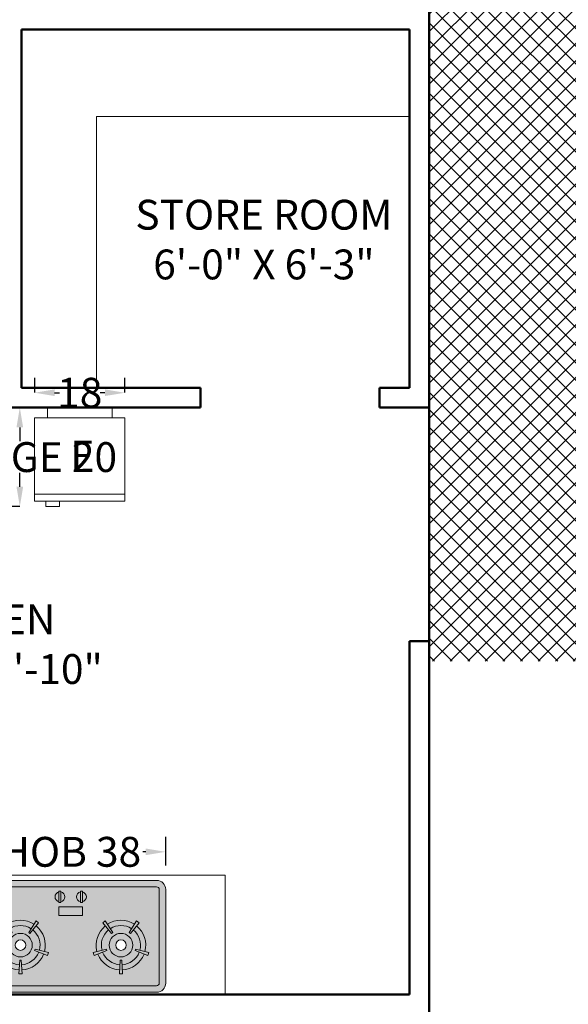
# Model space of a CAD drawing. Units: inches. Extents: x -466983 to 1020, y 324 to 318697.
# Tile 8 of 97: x 530 to 641, y 629 to 827. Entities that reach past the tile are written whole.
import ezdxf

# ---------------------------------------------------------------- set-up
doc = ezdxf.new("R2010")
doc.units = ezdxf.units.IN
doc.header["$MEASUREMENT"] = 0
for name, color, linetype, lineweight in [('A-ANNO-DIMS', 2, 'Continuous', 18), ('A-ANNO-TEXT', 7, 'Continuous', 18), ('A-AREA-IDEN', 7, 'Continuous', 25), ('A-EQPM', 8, 'Continuous', 18), ('A-FLOR-FIXT', 9, 'Continuous', 18), ('A-FLOR-PATT', 252, 'Continuous', 13), ('A-WALL', 7, 'Continuous', 50)]:
    doc.layers.add(name, color=color, linetype=linetype, lineweight=lineweight)
doc.styles.get("Standard").update_dxf_attribs({"font": 'arial.ttf'})
doc.dimstyles.get("Standard").update_dxf_attribs({"dimtxt": 6, "dimasz": 4, "dimexe": 3, "dimexo": 3, "dimgap": 0.09, "dimtad": 0, "dimtih": 1, "dimtoh": 1, "dimdec": 1, "dimzin": 0, "dimdsep": 46, "dimlunit": 3, "dimtxsty": 'Standard', "dimcen": 0.09, "dimadec": 0, "dimazin": 0, "dimtfac": 1, "dimtdec": 1, "dimtofl": 0, "dimtmove": 0, "dimatfit": 3, "dimfxl": 1, "dimtolj": 1, "dimtzin": 0, "dimarcsym": 0})

# ---------------------------------------------------------------- blocks, each defined once
blk = doc.blocks.new('Gas Stove')
h = blk.add_hatch(color=256)
h.dxf.hatch_style = 1
h.paths.add_polyline_path([(13032.81, 10915.17, 0.414214), (13029.34, 10918.64), (12963.86, 10918.64, 0.414214), (12960.39, 10915.17), (12960.39, 10879.45, 0.414214), (12963.86, 10875.98), (13029.34, 10875.98, 0.414214), (13032.81, 10879.45)])
h.paths.add_polyline_path([(13030.33, 10879.45, -0.414214), (13029.34, 10878.46), (12963.86, 10878.46, -0.414214), (12962.87, 10879.45), (12962.87, 10915.17, -0.414214), (12963.86, 10916.16), (13029.34, 10916.16, -0.414214), (13030.33, 10915.17)], flags=16)
h.paths.add_polyline_path([(13026, 10904.63), (13026.36, 10903.5), (13024.89, 10903.11, -0.295473), (13021.71, 10893.34), (13022.68, 10892.15), (13021.71, 10891.45), (13020.89, 10892.74, -0.295473), (13010.61, 10892.74), (13009.78, 10891.45), (13008.82, 10892.15), (13009.79, 10893.34, -0.295473), (13006.61, 10903.11), (13005.13, 10903.5), (13005.5, 10904.63), (13006.93, 10904.08, -0.295473), (13015.24, 10910.12), (13015.15, 10911.64), (13016.34, 10911.64), (13016.26, 10910.12, -0.295473), (13024.57, 10904.08)], flags=0)
h.paths.add_polyline_path([(13020.24, 10900.68, -1), (13011.25, 10900.68, -1)], flags=0)
h.paths.add_polyline_path([(13017.76, 10900.68, -1), (13013.73, 10900.68, -1)], flags=0)
h.paths.add_polyline_path([(13001.07, 10889.32), (13001.07, 10886.1), (12992.13, 10886.1), (12992.13, 10889.32)], flags=0)
h.paths.add_polyline_path([(13001.08, 10880.42), (13001.08, 10880.13), (13000.33, 10880.13), (13000.33, 10880.42, -0.820702), (13000.33, 10884.1), (13000.33, 10884.41), (13001.08, 10884.41), (13001.08, 10884.1, -0.816133)], flags=0)
h.paths.add_polyline_path([(12988.06, 10903.5), (12986.59, 10903.11, -0.295473), (12983.41, 10893.34), (12984.38, 10892.15), (12983.41, 10891.45), (12982.59, 10892.74, -0.295473), (12972.31, 10892.74), (12971.48, 10891.45), (12970.52, 10892.15), (12971.49, 10893.34, -0.295473), (12968.31, 10903.11), (12966.83, 10903.5), (12967.2, 10904.63), (12968.63, 10904.08, -0.295473), (12976.94, 10910.12), (12976.85, 10911.64), (12978.04, 10911.64), (12977.96, 10910.12, -0.295473), (12986.27, 10904.08), (12987.7, 10904.63)], flags=0)
h.paths.add_polyline_path([(12992.89, 10880.42), (12992.89, 10880.13), (12992.14, 10880.13), (12992.14, 10880.42, -0.816133), (12992.14, 10884.1), (12992.14, 10884.41), (12992.89, 10884.41), (12992.89, 10884.1, -0.820702)], flags=0)
h.paths.add_polyline_path([(12981.94, 10900.68, -1), (12972.95, 10900.68, -1)], flags=0)
h.paths.add_polyline_path([(12979.46, 10900.68, -1), (12975.43, 10900.68, -1)], flags=0)
h = blk.add_hatch(color=0)
h.dxf.hatch_style = 1
h.set_gradient(color1=(192, 192, 192), color2=(0, 0, 0))
h.paths.add_polyline_path([(13030.33, 10915.17, 0.414214), (13029.34, 10916.16), (12963.86, 10916.16, 0.414214), (12962.87, 10915.17), (12962.87, 10879.45, 0.414214), (12963.86, 10878.46), (13029.34, 10878.46, 0.414214), (13030.33, 10879.45)])
h.paths.add_polyline_path([(12987.7, 10904.63), (12988.06, 10903.5), (12986.59, 10903.11, -0.295473), (12983.41, 10893.34), (12984.38, 10892.15), (12983.41, 10891.45), (12982.59, 10892.74, -0.295473), (12972.31, 10892.74), (12971.48, 10891.45), (12970.52, 10892.15), (12971.49, 10893.34, -0.295473), (12968.31, 10903.11), (12966.83, 10903.5), (12967.2, 10904.63), (12968.63, 10904.08, -0.295473), (12976.94, 10910.12), (12976.85, 10911.64), (12978.04, 10911.64), (12977.96, 10910.12, -0.295473), (12986.27, 10904.08)], flags=16)
h.paths.add_polyline_path([(13005.5, 10904.63), (13006.93, 10904.08, -0.295473), (13015.24, 10910.12), (13015.15, 10911.64), (13016.34, 10911.64), (13016.26, 10910.12, -0.295473), (13024.57, 10904.08), (13026, 10904.63), (13026.36, 10903.5), (13024.89, 10903.11, -0.295473), (13021.71, 10893.34), (13022.68, 10892.15), (13021.71, 10891.45), (13020.89, 10892.74, -0.295473), (13010.61, 10892.74), (13009.78, 10891.45), (13008.82, 10892.15), (13009.79, 10893.34, -0.295473), (13006.61, 10903.11), (13005.13, 10903.5)], flags=16)
h.paths.add_polyline_path([(12981.94, 10900.68, -1), (12972.95, 10900.68, -1)], flags=0)
h.paths.add_polyline_path([(12979.46, 10900.68, -1), (12975.43, 10900.68, -1)], flags=0)
h.paths.add_polyline_path([(13020.24, 10900.68, -1), (13011.25, 10900.68, -1)], flags=0)
h.paths.add_polyline_path([(13017.76, 10900.68, -1), (13013.73, 10900.68, -1)], flags=0)
h.paths.add_polyline_path([(13001.07, 10889.32), (13001.07, 10886.1), (12992.13, 10886.1), (12992.13, 10889.32)], flags=16)
h.paths.add_polyline_path([(12992.89, 10884.41), (12992.89, 10884.1, -0.820702), (12992.89, 10880.42), (12992.89, 10880.13), (12992.14, 10880.13), (12992.14, 10880.42, -0.816133), (12992.14, 10884.1), (12992.14, 10884.41)], flags=16)
h.paths.add_polyline_path([(13000.33, 10884.41), (13001.08, 10884.41), (13001.08, 10884.1, -0.816133), (13001.08, 10880.42), (13001.08, 10880.13), (13000.33, 10880.13), (13000.33, 10880.42, -0.820702), (13000.33, 10884.1)], flags=16)
h.paths.add_polyline_path([(13022.97, 10902.61), (13021.31, 10902.17), (13021.12, 10902.73), (13022.72, 10903.36, 0.295997), (13016.14, 10908.14), (13016.04, 10906.42), (13015.45, 10906.42), (13015.35, 10908.14, 0.295997), (13008.78, 10903.36), (13010.38, 10902.73), (13010.19, 10902.17), (13008.53, 10902.61, 0.295997), (13011.04, 10894.87), (13012.13, 10896.2), (13012.61, 10895.85), (13011.68, 10894.41, 0.295997), (13019.82, 10894.41), (13018.89, 10895.85), (13019.37, 10896.2), (13020.45, 10894.87, 0.295997)], flags=0)
h = blk.add_hatch(color=256)
h.dxf.hatch_style = 1
h.set_gradient(color1=(237, 238, 153), color2=(128, 128, 128), name='INVSPHERICAL')
h.paths.add_polyline_path([(13030.33, 10915.17, 0.414214), (13029.34, 10916.16), (12963.86, 10916.16, 0.414214), (12962.87, 10915.17), (12962.87, 10879.45, 0.414214), (12963.86, 10878.46), (13029.34, 10878.46, 0.414214), (13030.33, 10879.45)])
h.paths.add_polyline_path([(12986.27, 10904.08), (12987.7, 10904.63), (12988.06, 10903.5), (12986.59, 10903.11, -0.295473), (12983.41, 10893.34), (12984.38, 10892.15), (12983.41, 10891.45), (12982.59, 10892.74, -0.295473), (12972.31, 10892.74), (12971.48, 10891.45), (12970.52, 10892.15), (12971.49, 10893.34, -0.295473), (12968.31, 10903.11), (12966.83, 10903.5), (12967.2, 10904.63), (12968.63, 10904.08, -0.295473), (12976.94, 10910.12), (12976.85, 10911.64), (12978.04, 10911.64), (12977.96, 10910.12, -0.295473)], flags=16)
h.paths.add_polyline_path([(12981.94, 10900.68, -1), (12972.95, 10900.68, -1)], flags=0)
h.paths.add_polyline_path([(12979.46, 10900.68, -1), (12975.43, 10900.68, -1)], flags=0)
h.paths.add_polyline_path([(13005.5, 10904.63), (13006.93, 10904.08, -0.295473), (13015.24, 10910.12), (13015.15, 10911.64), (13016.34, 10911.64), (13016.26, 10910.12, -0.295473), (13024.57, 10904.08), (13026, 10904.63), (13026.36, 10903.5), (13024.89, 10903.11, -0.295473), (13021.71, 10893.34), (13022.68, 10892.15), (13021.71, 10891.45), (13020.89, 10892.74, -0.295473), (13010.61, 10892.74), (13009.78, 10891.45), (13008.82, 10892.15), (13009.79, 10893.34, -0.295473), (13006.61, 10903.11), (13005.13, 10903.5)], flags=16)
h.paths.add_polyline_path([(12992.13, 10889.32), (13001.07, 10889.32), (13001.07, 10886.1), (12992.13, 10886.1)], flags=16)
h.paths.add_polyline_path([(13020.24, 10900.68, -1), (13011.25, 10900.68, -1)], flags=0)
h.paths.add_polyline_path([(13017.76, 10900.68, -1), (13013.73, 10900.68, -1)], flags=0)
h.paths.add_polyline_path([(12992.14, 10884.41), (12992.89, 10884.41), (12992.89, 10884.1, -0.820702), (12992.89, 10880.42), (12992.89, 10880.13), (12992.14, 10880.13), (12992.14, 10880.42, -0.816133), (12992.14, 10884.1)], flags=16)
h.paths.add_polyline_path([(13000.33, 10884.41), (13001.08, 10884.41), (13001.08, 10884.1, -0.816133), (13001.08, 10880.42), (13001.08, 10880.13), (13000.33, 10880.13), (13000.33, 10880.42, -0.820702), (13000.33, 10884.1)], flags=16)
h = blk.add_hatch(color=256)
h.dxf.hatch_style = 1
h.paths.add_polyline_path([(13005.5, 10904.63), (13005.13, 10903.5), (13010.19, 10902.17), (13010.38, 10902.73)])
h.paths.add_polyline_path([(13012.61, 10895.85), (13012.13, 10896.2), (13008.82, 10892.15), (13009.78, 10891.45)])
h.paths.add_polyline_path([(13019.37, 10896.2), (13018.89, 10895.85), (13021.71, 10891.45), (13022.68, 10892.15)])
h.paths.add_polyline_path([(13026.36, 10903.5), (13026, 10904.63), (13021.12, 10902.73), (13021.31, 10902.17)])
h.paths.add_polyline_path([(13016.34, 10911.64), (13015.15, 10911.64), (13015.45, 10906.42), (13016.04, 10906.42)])
h.paths.add_polyline_path([(12988.06, 10903.5), (12987.7, 10904.63), (12982.82, 10902.73), (12983.01, 10902.17)])
h.paths.add_polyline_path([(12978.04, 10911.64), (12976.85, 10911.64), (12977.15, 10906.42), (12977.74, 10906.42)])
h.paths.add_polyline_path([(12981.07, 10896.2), (12980.59, 10895.85), (12983.41, 10891.45), (12984.38, 10892.15)])
h.paths.add_polyline_path([(12974.31, 10895.85), (12973.83, 10896.2), (12970.52, 10892.15), (12971.48, 10891.45)])
h.paths.add_polyline_path([(12967.2, 10904.63), (12966.83, 10903.5), (12971.89, 10902.17), (12972.08, 10902.73)])
h = blk.add_hatch(color=256)
h.dxf.hatch_style = 1
h.paths.add_polyline_path([(12986.59, 10903.11), (12984.67, 10902.61, -0.295997), (12982.15, 10894.87), (12983.41, 10893.34, 0.295473)])
h.paths.add_polyline_path([(12977.96, 10910.12), (12977.84, 10908.14, -0.295997), (12984.42, 10903.36), (12986.27, 10904.08, 0.295473)])
h.paths.add_polyline_path([(12977.06, 10908.14), (12976.94, 10910.12, 0.295473), (12968.63, 10904.08), (12970.48, 10903.36, -0.295997)])
h.paths.add_polyline_path([(12970.23, 10902.61), (12968.31, 10903.11, 0.295473), (12971.49, 10893.34), (12972.75, 10894.87, -0.295997)])
h.paths.add_polyline_path([(12982.59, 10892.74), (12981.52, 10894.41, -0.295997), (12973.38, 10894.41), (12972.31, 10892.74, 0.295473)])
h.paths.add_polyline_path([(13016.26, 10910.12), (13016.14, 10908.14, -0.295997), (13022.72, 10903.36), (13024.57, 10904.08, 0.295473)])
h.paths.add_polyline_path([(13024.89, 10903.11), (13022.97, 10902.61, -0.295997), (13020.45, 10894.87), (13021.71, 10893.34, 0.295473)])
h.paths.add_polyline_path([(13020.89, 10892.74), (13019.82, 10894.41, -0.295997), (13011.68, 10894.41), (13010.61, 10892.74, 0.295473)])
h.paths.add_polyline_path([(13008.53, 10902.61), (13006.61, 10903.11, 0.295473), (13009.79, 10893.34), (13011.04, 10894.87, -0.295997)])
h.paths.add_polyline_path([(13015.35, 10908.14), (13015.24, 10910.12, 0.295473), (13006.93, 10904.08), (13008.78, 10903.36, -0.295997)])
h = blk.add_hatch(color=0)
h.dxf.hatch_style = 1
h.set_gradient(color1=(192, 192, 192), color2=(0, 0, 0), name='CYLINDER')
h.paths.add_polyline_path([(13022.97, 10902.61), (13021.31, 10902.17), (13021.12, 10902.73), (13022.72, 10903.36, 0.295997), (13016.14, 10908.14), (13016.04, 10906.42), (13015.45, 10906.42), (13015.35, 10908.14, 0.295997), (13008.78, 10903.36), (13010.38, 10902.73), (13010.19, 10902.17), (13008.53, 10902.61, 0.295997), (13011.04, 10894.87), (13012.13, 10896.2), (13012.61, 10895.85), (13011.68, 10894.41, 0.295997), (13019.82, 10894.41), (13018.89, 10895.85), (13019.37, 10896.2), (13020.45, 10894.87, 0.295997)])
h.paths.add_polyline_path([(13011.25, 10900.68, -1), (13020.24, 10900.68, -1)], flags=16)
h.paths.add_polyline_path([(13013.73, 10900.68, -1), (13017.76, 10900.68, -1)], flags=0)
h.paths.add_polyline_path([(12984.67, 10902.61), (12983.01, 10902.17), (12982.82, 10902.73), (12984.42, 10903.36, 0.295997), (12977.84, 10908.14), (12977.74, 10906.42), (12977.15, 10906.42), (12977.06, 10908.14, 0.295997), (12970.48, 10903.36), (12972.08, 10902.73), (12971.89, 10902.17), (12970.23, 10902.61, 0.295997), (12972.75, 10894.87), (12973.83, 10896.2), (12974.31, 10895.85), (12973.38, 10894.41, 0.295997), (12981.52, 10894.41), (12980.59, 10895.85), (12981.07, 10896.2), (12982.15, 10894.87, 0.295997)])
h.paths.add_polyline_path([(12972.95, 10900.68, -1), (12981.94, 10900.68, -1)], flags=16)
h.paths.add_polyline_path([(12975.43, 10900.68, -1), (12979.46, 10900.68, -1)], flags=0)
h = blk.add_hatch(color=0)
h.dxf.hatch_style = 1
h.set_gradient(color1=(0, 0, 255), color2=(255, 0, 0), name='CYLINDER')
h.paths.add_polyline_path([(13011.25, 10900.68, 1), (13020.24, 10900.68, 1)])
h.paths.add_polyline_path([(13017.76, 10900.68, -1), (13013.73, 10900.68, -1)], flags=16)
h.paths.add_polyline_path([(12972.95, 10900.68, 1), (12981.94, 10900.68, 1)])
h.paths.add_polyline_path([(12979.46, 10900.68, -1), (12975.43, 10900.68, -1)], flags=16)
h = blk.add_hatch(color=256)
h.dxf.hatch_style = 1
h.paths.add_polyline_path([(13001.07, 10889.32), (12992.13, 10889.32), (12992.13, 10886.1), (13001.07, 10886.1)])
h.paths.add_polyline_path([(13001.08, 10884.41), (13000.33, 10884.41), (13000.33, 10880.13), (13001.08, 10880.13)])
h.paths.add_polyline_path([(12992.89, 10884.41), (12992.14, 10884.41), (12992.14, 10880.13), (12992.89, 10880.13)])
h = blk.add_hatch(color=0)
h.dxf.hatch_style = 1
h.set_gradient(color1=(0, 0, 255), color2=(255, 0, 0), name='CYLINDER')
h.paths.add_polyline_path([(13001.08, 10884.1), (13001.08, 10880.42, 0.816133)])
h.paths.add_polyline_path([(13000.33, 10884.1, 0.820702), (13000.33, 10880.42)])
h.paths.add_polyline_path([(12992.89, 10884.1), (12992.89, 10880.42, 0.820702)])
h.paths.add_polyline_path([(12992.14, 10884.1, 0.816133), (12992.14, 10880.42)])
at = {"color": 0}
for p, q in [((12963.86, 10918.64), (13029.34, 10918.64)), ((12960.39, 10879.45), (12960.39, 10915.17)), ((12962.87, 10879.45), (12962.87, 10915.17)), ((12963.86, 10916.16), (13029.34, 10916.16)), ((13030.33, 10915.17), (13030.33, 10879.45)), ((13032.81, 10915.17), (13032.81, 10879.45)), ((12976.85, 10911.64), (12977.15, 10906.42)), ((12976.85, 10911.64), (12978.04, 10911.64)), ((12978.04, 10911.64), (12977.74, 10906.42)), ((13015.15, 10911.64), (13015.45, 10906.42)), ((13016.34, 10911.64), (13015.15, 10911.64)), ((13016.34, 10911.64), (13016.04, 10906.42)), ((12977.15, 10906.42), (12977.74, 10906.42)), ((13016.04, 10906.42), (13015.45, 10906.42)), ((12966.83, 10903.5), (12967.2, 10904.63)), ((12966.83, 10903.5), (12971.89, 10902.17)), ((12967.2, 10904.63), (12972.08, 10902.73)), ((12971.89, 10902.17), (12972.08, 10902.73)), ((12987.7, 10904.63), (12982.82, 10902.73)), ((12982.82, 10902.73), (12983.01, 10902.17)), ((12988.06, 10903.5), (12983.01, 10902.17)), ((12987.7, 10904.63), (12988.06, 10903.5)), ((13005.5, 10904.63), (13005.13, 10903.5)), ((13005.13, 10903.5), (13010.19, 10902.17)), ((13005.5, 10904.63), (13010.38, 10902.73)), ((13010.38, 10902.73), (13010.19, 10902.17)), ((13026, 10904.63), (13021.12, 10902.73)), ((13021.31, 10902.17), (13021.12, 10902.73)), ((13026.36, 10903.5), (13021.31, 10902.17)), ((13026.36, 10903.5), (13026, 10904.63)), ((12970.52, 10892.15), (12973.83, 10896.2)), ((12971.48, 10891.45), (12974.31, 10895.85)), ((12974.31, 10895.85), (12973.83, 10896.2)), ((12981.07, 10896.2), (12980.59, 10895.85)), ((12983.41, 10891.45), (12980.59, 10895.85)), ((12984.38, 10892.15), (12981.07, 10896.2)), ((13008.82, 10892.15), (13012.13, 10896.2)), ((13009.78, 10891.45), (13012.61, 10895.85)), ((13012.13, 10896.2), (13012.61, 10895.85)), ((13018.89, 10895.85), (13019.37, 10896.2)), ((13021.71, 10891.45), (13018.89, 10895.85)), ((13022.68, 10892.15), (13019.37, 10896.2)), ((12971.48, 10891.45), (12970.52, 10892.15)), ((12984.38, 10892.15), (12983.41, 10891.45)), ((13008.82, 10892.15), (13009.78, 10891.45)), ((13021.71, 10891.45), (13022.68, 10892.15)), ((12992.13, 10889.32), (12992.13, 10886.1)), ((13001.07, 10889.32), (12992.13, 10889.32)), ((13001.07, 10886.1), (13001.07, 10889.32)), ((12992.13, 10886.1), (13001.07, 10886.1)), ((12992.14, 10884.41), (12992.14, 10880.13)), ((12992.89, 10884.41), (12992.14, 10884.41)), ((12992.89, 10880.13), (12992.89, 10884.41)), ((13000.33, 10884.41), (13001.08, 10884.41)), ((13000.33, 10880.13), (13000.33, 10884.41)), ((13001.08, 10884.41), (13001.08, 10880.13)), ((12992.14, 10880.13), (12992.89, 10880.13)), ((13001.08, 10880.13), (13000.33, 10880.13)), ((13029.34, 10878.46), (12963.86, 10878.46)), ((13029.34, 10875.98), (12963.86, 10875.98))]:
    blk.add_line(p, q, dxfattribs=at)
for centre, radius in [((12977.45, 10900.68), 4.49), ((12977.45, 10900.68), 2.01), ((13015.75, 10900.68), 4.49), ((13015.75, 10900.68), 2.01)]:
    blk.add_circle(centre, radius, dxfattribs=at)
for centre, radius, start, end in [((12963.86, 10915.17), 3.47, 90, 180), ((13029.34, 10915.17), 3.47, 0, 90), ((12963.86, 10915.17), 0.992, 90, 180), ((13029.34, 10915.17), 0.992, 0, 90), ((12977.45, 10900.68), 9.46, 93.078, 158.922), ((12977.45, 10900.68), 9.46, 21.078, 86.922), ((13015.75, 10900.68), 9.46, 93.078, 158.922), ((13015.75, 10900.68), 9.46, 21.078, 86.922), ((12977.45, 10900.68), 7.47, 93.0228, 158.9772), ((12977.45, 10900.68), 7.47, 21.0228, 86.9772), ((13015.75, 10900.68), 7.47, 93.0228, 158.9772), ((13015.75, 10900.68), 7.47, 21.0228, 86.9772), ((12977.45, 10900.68), 9.46, 165.078, 230.922), ((12977.45, 10900.68), 7.47, 165.0228, 230.9772), ((12977.45, 10900.68), 7.47, 309.0228, 14.9772), ((12977.45, 10900.68), 9.46, 309.078, 14.922), ((13015.75, 10900.68), 9.46, 165.078, 230.922), ((13015.75, 10900.68), 7.47, 165.0228, 230.9772), ((13015.75, 10900.68), 7.47, 309.0228, 14.9772), ((13015.75, 10900.68), 9.46, 309.078, 14.922), ((12977.45, 10900.68), 9.46, 237.078, 302.922), ((12977.45, 10900.68), 7.47, 237.0228, 302.9772), ((13015.75, 10900.68), 9.46, 237.078, 302.922), ((13015.75, 10900.68), 7.47, 237.0228, 302.9772), ((12992.52, 10882.26), 1.88, 101.5619, 258.4381), ((12992.52, 10882.26), 1.88, 281.2484, 78.7516), ((13000.7, 10882.26), 1.88, 101.2484, 258.7516), ((13000.7, 10882.26), 1.88, 281.5619, 78.4381), ((12963.86, 10879.45), 3.47, 180, 270), ((12963.86, 10879.45), 0.992, 180, 270), ((13029.34, 10879.45), 0.992, 270, 0), ((13029.34, 10879.45), 3.47, 270, 0)]:
    blk.add_arc(centre, radius, start, end, dxfattribs=at)
blk = doc.blocks.new('A$C659B0DF6')
for p, q in [((423, 642.1), (423, 606.1)), ((513, 642.1), (423, 642.1)), ((513, 606.1), (513, 642.1)), ((585, 606.1), (0, 606.1)), ((0, 66.1), (0, 606.1)), ((585, 66.1), (585, 606.1)), ((585, 561.1), (0, 561.1)), ((0, 66.1), (585, 66.1)), ((82.3, 0), (82.3, 66.1)), ((502.7, 0), (502.7, 66.1)), ((82.3, 0), (502.7, 0))]:
    blk.add_line(p, q)
blk = doc.blocks.new('*D107')
at = {"layer": 'A-ANNO-DIMS', "color": 0, "lineweight": -2, "transparency": 16777216}
for p, q in [((521.6, 656.87), (521.6, 662.6)), ((559.81, 656.87), (559.81, 662.6)), ((525.6, 659.6), (526.23, 659.6)), ((555.81, 659.6), (555.18, 659.6))]:
    blk.add_line(p, q, dxfattribs=at)
at = {"layer": 'A-ANNO-DIMS', "color": 0, "transparency": 16777216}
for points in [[(525.6, 660.27), (525.6, 658.93), (521.6, 659.6)], [(555.81, 660.27), (555.81, 658.93), (559.81, 659.6)]]:
    blk.add_solid(points, dxfattribs=at)
at = {"layer": 'Defpoints', "color": 0, "transparency": 16777216}
for p in [(521.6, 659.6), (521.6, 653.87), (559.81, 653.87)]:
    blk.add_point(p, dxfattribs=at)
at = {"layer": 'A-ANNO-DIMS', "color": 0, "transparency": 16777216, "insert": (540.71, 659.6), "char_height": 6, "attachment_point": 5}
blk.add_mtext('\\A1;HOB 38', dxfattribs=at)
blk = doc.blocks.new('*D109')
at = {"layer": 'A-ANNO-DIMS', "color": 0, "lineweight": -2, "transparency": 16777216}
for p, q in [((530.46, 748.94), (527.47, 748.94)), ((530.47, 744.94), (530.47, 742.17)), ((530.47, 733.02), (530.47, 735.79)), ((530.46, 729.02), (527.47, 729.02))]:
    blk.add_line(p, q, dxfattribs=at)
at = {"layer": 'A-ANNO-DIMS', "color": 0, "transparency": 16777216}
for points in [[(529.8, 744.94), (531.14, 744.94), (530.47, 748.94)], [(529.8, 733.02), (531.14, 733.02), (530.47, 729.02)]]:
    blk.add_solid(points, dxfattribs=at)
at = {"layer": 'Defpoints', "color": 0, "transparency": 16777216}
for p in [(533.46, 748.94), (530.47, 729.02), (533.46, 729.02)]:
    blk.add_point(p, dxfattribs=at)
at = {"layer": 'A-ANNO-DIMS', "color": 0, "transparency": 16777216, "insert": (530.47, 738.98), "char_height": 6, "attachment_point": 5}
blk.add_mtext('\\A1;FRIDGE 20', dxfattribs=at)
blk = doc.blocks.new('*D110')
at = {"layer": 'A-ANNO-DIMS', "color": 0, "lineweight": -2, "transparency": 16777216}
for p, q in [((533.46, 751.94), (533.46, 754.92)), ((551.6, 751.94), (551.6, 754.92)), ((537.46, 751.92), (538.42, 751.92)), ((547.6, 751.92), (546.64, 751.92))]:
    blk.add_line(p, q, dxfattribs=at)
at = {"layer": 'A-ANNO-DIMS', "color": 0, "transparency": 16777216}
for points in [[(537.46, 752.59), (537.46, 751.26), (533.46, 751.92)], [(547.6, 752.59), (547.6, 751.26), (551.6, 751.92)]]:
    blk.add_solid(points, dxfattribs=at)
at = {"layer": 'Defpoints', "color": 0, "transparency": 16777216}
for p in [(533.46, 751.92), (533.46, 748.94), (551.6, 748.94)]:
    blk.add_point(p, dxfattribs=at)
at = {"layer": 'A-ANNO-DIMS', "color": 0, "transparency": 16777216, "insert": (542.53, 751.92), "char_height": 6, "attachment_point": 5}
blk.add_mtext('\\A1;18', dxfattribs=at)

msp = doc.modelspace()

# ---------------------------------------------------------------- hatches: boundary and pattern name
at = {"layer": 'A-FLOR-PATT', "transparency": 33554572}
h = msp.add_hatch(dxfattribs=at)
h.set_pattern_fill('ANSI37', color=256, scale=30)
h.set_pattern_definition([(45, (-1212.4137, -290.035), (-2.6516504, 2.6516504), []), (135, (-1212.4137, -290.035), (-2.6516504, -2.6516504), [])])
h.paths.add_polyline_path([(901.81, 1075.94), (900.61, 1075.94), (900.61, 1065.39), (899.39, 1065.39), (898.09, 1065.39), (892.84, 1058.71, -0.258377), (892.19, 1058.35), (879.98, 1058.35, -0.20177), (879.44, 1058.58), (874.08, 1065.39), (872.78, 1065.39), (871.56, 1065.39), (871.56, 1075.94), (813.81, 1075.94), (813.81, 1044.79), (832.39, 1044.79, -0.394795), (848.66, 1028.54), (848.66, 1009.94), (901.81, 1009.94), (901.81, 1015.94), (901.31, 1015.94), (871.31, 1015.94), (871.31, 1017.25), (871.33, 1017.25, -0.401453), (901.31, 1045.94), (901.81, 1045.94)])
edge = h.paths.add_edge_path(flags=16)
edge.add_line((847.77, 1068.95), (847.77, 1073.71))
edge.add_arc((849.23, 1073.71), 1.45, 90, 180, ccw=False)
edge.add_line((849.23, 1075.16), (864.49, 1075.16))
edge.add_arc((864.49, 1073.71), 1.45, 0, 90, ccw=False)
edge.add_line((865.95, 1073.71), (865.95, 1069))
edge.add_arc((832.64, 1068.98), 33.3, -20.6123, 0.0472, ccw=False)
edge.add_ellipse((856.86, 1058.48), major_axis=(0, 10.21), ratio=0.685919, start_angle=100.0088, end_angle=259.9912, ccw=False)
edge.add_arc((881.07, 1068.98), 33.3, 180.0472, 200.6123, ccw=False)
h.paths.add_polyline_path([(853.15, 1066.48), (853.15, 1066.45), (853.15, 1066.45, 0.433107), (852.92, 1066.68), (852.92, 1066.45), (853.15, 1066.45), (853.15, 1066.48), (853.09, 1066.61, 0.697939), (852.7, 1066.45), (852.7, 1066.45), (852.7, 1066.48), (852.92, 1067), (852.92, 1066.68, -0.396254)], flags=0)
h.paths.add_polyline_path([(861.02, 1066.48), (861.02, 1066.45), (861.02, 1066.45, 0.416404), (860.8, 1066.68), (860.8, 1066.45), (861.02, 1066.45), (861.02, 1066.48), (860.97, 1066.61, 0.713344), (860.57, 1066.45), (860.57, 1066.45), (860.57, 1066.48), (860.8, 1067), (860.8, 1066.68, -0.379973)], flags=0)
edge = h.paths.add_edge_path(flags=0)
edge.add_spline(control_points=[(861.13, 1065.79), (861.47, 1065.25), (861.61, 1065.02), (861.98, 1064.37), (862.19, 1063.94), (862.56, 1063.04), (862.72, 1062.56), (862.99, 1061.58), (863.09, 1061.07), (863.25, 1060.03), (863.29, 1059.5), (863.33, 1058.44), (863.32, 1057.91), (863.24, 1056.85), (863.17, 1056.33), (862.97, 1055.31), (862.84, 1054.81), (862.54, 1053.85), (862.36, 1053.39), (861.95, 1052.52), (861.73, 1052.12), (861.23, 1051.36), (860.97, 1051.02), (860.4, 1050.39), (860.11, 1050.12), (859.49, 1049.65), (859.18, 1049.45), (858.53, 1049.13), (858.2, 1049.01), (857.53, 1048.85), (857.2, 1048.81), (856.52, 1048.81), (856.19, 1048.85), (855.52, 1049.01), (855.19, 1049.13), (854.54, 1049.45), (854.23, 1049.64), (853.61, 1050.12), (853.32, 1050.39), (852.75, 1051.01), (852.49, 1051.36), (852, 1052.11), (851.77, 1052.52), (851.36, 1053.39), (851.18, 1053.85), (850.88, 1054.81), (850.75, 1055.31), (850.55, 1056.33), (850.48, 1056.85), (850.4, 1057.9), (850.39, 1058.44), (850.43, 1059.5), (850.47, 1060.03), (850.63, 1061.07), (850.73, 1061.58), (851, 1062.56), (851.16, 1063.04), (851.53, 1063.94), (851.73, 1064.37), (852.11, 1065.02), (852.25, 1065.25), (852.61, 1065.73)], knot_values=[3.915332, 3.915332, 3.915332, 3.915332, 4.013468, 4.013468, 4.175532, 4.175532, 4.337596, 4.337596, 4.49966, 4.49966, 4.661724, 4.661724, 4.823788, 4.823788, 4.985852, 4.985852, 5.147916, 5.147916, 5.30998, 5.30998, 5.472044, 5.472044, 5.634109, 5.634109, 5.796173, 5.796173, 5.958237, 5.958237, 6.120301, 6.120301, 6.282365, 6.282365, 6.444429, 6.444429, 6.606493, 6.606493, 6.768557, 6.768557, 6.930621, 6.930621, 7.092685, 7.092685, 7.254749, 7.254749, 7.416813, 7.416813, 7.578878, 7.578878, 7.740942, 7.740942, 7.903006, 7.903006, 8.06507, 8.06507, 8.227134, 8.227134, 8.389198, 8.389198, 8.551262, 8.551262, 8.65037, 8.65037, 8.65037, 8.65037], degree=3, periodic=0)
edge.add_line((852.64, 1065.79), (861.13, 1065.79))
edge = h.paths.add_edge_path(flags=0)
edge.add_ellipse((856.85, 1057.74), major_axis=(0, 7.79), ratio=0.687861, start_angle=0, end_angle=360)
h.paths.add_polyline_path([(848.86, 1069.39), (848.86, 1073.96, -0.414214), (849.95, 1075.05), (863.77, 1075.05, -0.414214), (864.86, 1073.96), (864.86, 1069.39, -0.388936), (864.52, 1069.03, -0.043561), (849.2, 1069.03, -0.388936)], flags=0)
h.paths.add_polyline_path([(853.1, 1068.11, -1), (852.68, 1068.11, -1)], flags=0)
edge = h.paths.add_edge_path(flags=0)
edge.add_ellipse((856.86, 1057.34), major_axis=(0, 2.21), ratio=0.657164, start_angle=0, end_angle=360)
h.paths.add_polyline_path([(861.04, 1068.11, -1), (860.62, 1068.11, -1)], flags=0)
edge = h.paths.add_edge_path()
edge.add_line((573.95, 1057.34), (573.95, 1075.94))
edge.add_line((573.95, 1075.94), (558.73, 1075.94))
edge.add_line((558.73, 1075.94), (558.73, 1065.39))
edge.add_line((558.73, 1065.39), (557.51, 1065.39))
edge.add_line((557.51, 1065.39), (556.21, 1065.39))
edge.add_line((556.21, 1065.39), (550.95, 1058.71))
edge.add_arc((550.3, 1059.12), 0.765, 270, 327.9483, ccw=False)
edge.add_line((550.3, 1058.35), (538.1, 1058.35))
edge.add_arc((538.1, 1059.12), 0.765, 224.3704, 270, ccw=False)
edge.add_line((537.55, 1058.58), (532.2, 1065.39))
edge.add_line((532.2, 1065.39), (530.9, 1065.39))
edge.add_line((530.9, 1065.39), (529.67, 1065.39))
edge.add_line((529.67, 1065.39), (529.67, 1075.94))
edge.add_line((529.67, 1075.94), (520.81, 1075.94))
edge.add_line((520.81, 1075.94), (520.81, 1045.94))
edge.add_line((520.81, 1045.94), (521.31, 1045.94))
edge.add_arc((521.31, 1015.94), 30, 2.5075, 90, ccw=False)
edge.add_line((551.28, 1017.25), (551.31, 1017.25))
edge.add_line((551.31, 1017.25), (551.31, 1015.94))
edge.add_line((551.31, 1015.94), (520.81, 1015.94))
edge.add_line((520.81, 1015.94), (520.81, 1009.94))
edge.add_line((520.81, 1009.94), (559.19, 1010.4))
edge.add_arc((559.19, 1011.86), 1.45, 180, 270, ccw=False)
edge.add_line((557.74, 1011.86), (557.74, 1016.56))
edge.add_arc((591.04, 1016.59), 33.3, 159.3877, 180.0472, ccw=False)
edge.add_ellipse((566.82, 1027.08), major_axis=(0, 10.21), ratio=0.685919, start_angle=280.0088, end_angle=439.9912, ccw=False)
edge.add_arc((542.61, 1016.59), 33.3, 0.0472, 20.6123, ccw=False)
edge.add_line((575.91, 1016.62), (575.91, 1011.86))
edge.add_arc((574.46, 1011.86), 1.45, -90, 0, ccw=False)
edge.add_line((574.46, 1010.4), (608.81, 1009.94))
edge.add_line((608.81, 1009.94), (608.81, 1041.09))
edge.add_line((608.81, 1041.09), (590.22, 1041.09))
edge.add_arc((590.78, 1057.91), 16.83, 181.9277, 268.1032, ccw=False)
edge = h.paths.add_edge_path()
edge.add_ellipse((494.24, 583.62), major_axis=(0, 10.21), ratio=0.685919, start_angle=280.0088, end_angle=439.9912, ccw=False)
edge.add_arc((470.03, 573.12), 33.3, 0.0472, 20.6123, ccw=False)
edge.add_line((503.33, 573.15), (503.33, 568.39))
edge.add_arc((501.88, 568.39), 1.45, -90, 0, ccw=False)
edge.add_line((501.88, 566.94), (539.81, 566.94))
edge.add_line((539.81, 566.94), (539.81, 572.94))
edge.add_line((539.81, 572.94), (539.31, 572.94))
edge.add_line((539.31, 572.94), (509.31, 572.94))
edge.add_line((509.31, 572.94), (509.31, 574.25))
edge.add_line((509.31, 574.25), (509.33, 574.25))
edge.add_arc((539.31, 572.94), 30, 90, 177.4925, ccw=False)
edge.add_line((539.31, 602.94), (539.81, 602.94))
edge.add_line((539.81, 602.94), (539.81, 626.94))
edge.add_line((539.81, 626.94), (531.77, 626.94))
edge.add_line((531.77, 626.94), (531.77, 616.39))
edge.add_line((531.77, 616.39), (530.55, 616.39))
edge.add_line((530.55, 616.39), (529.25, 616.39))
edge.add_line((529.25, 616.39), (523.71, 609.35))
edge.add_line((523.71, 609.35), (510.78, 609.35))
edge.add_line((510.78, 609.35), (505.24, 616.39))
edge.add_line((505.24, 616.39), (503.94, 616.39))
edge.add_line((503.94, 616.39), (502.72, 616.39))
edge.add_line((502.72, 616.39), (502.72, 626.94))
edge.add_line((502.72, 626.94), (481.7, 626.94))
edge.add_line((481.7, 626.94), (481.7, 611))
edge.add_arc((467.27, 611.47), 14.44, 271.9277, 358.1032, ccw=False)
edge.add_line((467.76, 597.05), (451.81, 597.05))
edge.add_line((451.81, 597.05), (451.81, 584.4))
edge.add_line((451.81, 584.4), (451.81, 566.94))
edge.add_line((451.81, 566.94), (486.61, 566.94))
edge.add_arc((486.61, 568.39), 1.45, 180, 270, ccw=False)
edge.add_line((485.16, 568.39), (485.16, 573.1))
edge.add_arc((518.46, 573.12), 33.3, 159.3877, 180.0472, ccw=False)
h.paths.add_polyline_path([(836.26, 1020.73), (879.89, 1020.73), (879.89, 1039.39), (836.26, 1039.39)], flags=25)
h.paths.add_polyline_path([(549.99, 1036.75), (593.61, 1036.75), (593.61, 1055.41), (549.99, 1055.41)], flags=24)
h.paths.add_polyline_path([(475.12, 595.6), (518.75, 595.6), (518.75, 614.25), (475.12, 614.25)], flags=24)
h = msp.add_hatch(dxfattribs=at)
h.set_pattern_fill('ANSI37', color=256, scale=20)
h.set_pattern_definition([(45, (-1212.4137, -290.035), (-1.767767, 1.767767), []), (135, (-1212.4137, -290.035), (-1.767767, -1.767767), [])])
h.paths.add_polyline_path([(809.81, 870.94), (809.81, 888.15), (807, 888.15), (802.66, 888.15), (789.38, 888.15), (786.28, 888.15, -0.414214), (785.5, 888.94), (785.5, 900.2), (785.5, 908.47, -0.414214), (786.81, 909.78, -0.414214), (785.5, 911.09), (785.5, 929.1, -0.414214), (786.81, 930.41, -0.414214), (785.5, 931.72), (785.5, 931.9, -0.414214), (784.19, 930.59), (766.72, 930.59, -0.412359), (765.41, 931.9, -0.413741), (764.11, 930.58), (744.58, 930.42, -0.416556), (743.79, 931.21), (743.79, 933.52), (742.22, 933.52), (742.22, 952.02, -0.001344), (743.79, 952.2), (743.79, 953.94), (678.59, 953.94), (678.59, 951.13), (678.59, 946.79), (678.59, 933.52), (678.59, 930.42, -0.414214), (677.81, 929.63), (666.55, 929.63), (658.27, 929.63, -0.414214), (656.96, 930.94, -0.414214), (655.66, 929.63), (637.64, 929.63, -0.414214), (636.33, 930.94, -0.414214), (635.02, 929.63), (634.84, 929.63, -0.414214), (636.15, 928.32), (636.15, 910.85, -0.412359), (634.85, 909.55, -0.413741), (636.17, 908.25), (636.32, 888.71, -0.416556), (635.54, 887.92), (633.23, 887.92), (633.23, 886.35), (614.72, 886.35, -0.001344), (614.54, 887.92), (612.81, 887.92), (612.81, 834.94), (612.81, 752.94), (612.81, 748.94), (612.81, 697.94), (654.81, 697.94), (654.81, 701.94), (715.81, 701.94), (715.81, 737.44), (774.29, 737.44), (774.29, 795.94), (809.81, 795.94)])
h.paths.add_polyline_path([(679.28, 849.58, 0.102523), (682.15, 849.26, -0.080461), (694.54, 849.77, -0.283899), (694.48, 849.01, 0.136605), (694.41, 848.81, -0.030441), (694.54, 846.89), (694.54, 842.62), (694.54, 838.35, -0.028219), (694.42, 836.57), (694.43, 836.57, 0.196187), (694.45, 836.27, -0.302897), (694.54, 835.47, -0.080461), (682.15, 835.98, 0.102523), (679.28, 835.66, -0.58611), (678.65, 836.02), (678.65, 849.22, -0.58611)], flags=16)
h.paths.add_polyline_path([(679.52, 848.65, 0.699597), (679.48, 848.63, 1.20716), (679.19, 848.74, 0.010621)], flags=0)
h.paths.add_polyline_path([(679.49, 836.56, -0.013798), (679.92, 836.66, -0.071703), (682.85, 837.14, -0.165743), (682.17, 839.1), (682.17, 842.61), (682.17, 846.06, -0.240616), (683.47, 848.68, -0.068263), (693.93, 849.01), (693.79, 848.71), (693.79, 849.02, 0.067332), (683.47, 848.68, 0.240616), (682.17, 846.06), (682.17, 842.61), (682.17, 839.1, 0.23459), (683.46, 836.55, 0.068093), (693.79, 836.2), (693.79, 836.51), (693.93, 836.21, -0.077215), (682.24, 836.78, 0.086627), (679.53, 836.57, -0.628402), (679.5, 836.57), (679.5, 836.61, 0.910458)], flags=0)
h.paths.add_polyline_path([(679.48, 848.64), (679.21, 848.65), (679.21, 836.57, 0.913566), (679.36, 836.59), (679.48, 836.58)], flags=0)
h.paths.add_polyline_path([(679.28, 829.86, 0.102523), (682.15, 829.55, -0.080461), (694.54, 830.06, -0.283899), (694.48, 829.29, 0.136605), (694.41, 829.1, -0.030441), (694.54, 827.18), (694.54, 822.9), (694.54, 818.63, -0.028219), (694.42, 816.85), (694.43, 816.85, 0.196187), (694.45, 816.56, -0.302897), (694.54, 815.75, -0.080461), (682.15, 816.26, 0.102523), (679.28, 815.95, -0.58611), (678.65, 816.3), (678.65, 829.51, -0.58611)], flags=16)
h.paths.add_polyline_path([(679.52, 828.94, 0.699597), (679.48, 828.92, 1.20716), (679.19, 829.03, 0.010621)], flags=0)
h.paths.add_polyline_path([(679.49, 816.85, -0.013798), (679.92, 816.94, -0.071703), (682.85, 817.43, -0.165743), (682.17, 819.39), (682.17, 822.89), (682.17, 826.34, -0.240616), (683.47, 828.96, -0.068263), (693.93, 829.29), (693.79, 828.99), (693.79, 829.31, 0.067332), (683.47, 828.96, 0.240616), (682.17, 826.34), (682.17, 822.89), (682.17, 819.39, 0.23459), (683.46, 816.84, 0.068093), (693.79, 816.48), (693.79, 816.8), (693.93, 816.49, -0.077215), (682.24, 817.07, 0.086627), (679.53, 816.85, -0.628402), (679.5, 816.86), (679.5, 816.89, 0.910458)], flags=0)
h.paths.add_polyline_path([(679.48, 828.92), (679.21, 828.93), (679.21, 816.86, 0.913566), (679.36, 816.87), (679.48, 816.87)], flags=0)
h.paths.add_polyline_path([(679.28, 810.15, 0.102523), (682.15, 809.83, -0.080461), (694.54, 810.34, -0.3023), (694.45, 809.54, 0.10023), (694.41, 809.39, -0.03057), (694.54, 807.46), (694.54, 803.19), (694.54, 798.92, -0.03057), (694.41, 796.99, 0.10023), (694.45, 796.84, -0.3023), (694.54, 796.04, -0.080461), (682.15, 796.55, 0.102523), (679.28, 796.23, -0.58611), (678.65, 796.59), (678.65, 809.79, -0.58611)], flags=16)
h.paths.add_polyline_path([(679.52, 809.24, 0.699597), (679.48, 809.22, 1.20716), (679.19, 809.33, 0.010621)], flags=0)
h.paths.add_polyline_path([(679.49, 797.15, -0.013798), (679.92, 797.25, -0.071703), (682.85, 797.73, -0.165743), (682.17, 799.69), (682.17, 803.2), (682.17, 806.65, -0.239349), (683.46, 809.26, -0.072465), (694.45, 809.54, 0.197932), (694.43, 809.24), (693.79, 809.3), (693.79, 809.61, 0.068093), (683.46, 809.26, 0.239349), (682.17, 806.65), (682.17, 803.2), (682.17, 799.69, 0.235854), (683.47, 797.13, 0.067332), (693.79, 796.79), (693.79, 797.1), (694.43, 797.16, 0.197932), (694.45, 796.86, -0.080419), (682.16, 797.38, 0.083867), (679.53, 797.16, -0.628402), (679.5, 797.16), (679.5, 797.2, 0.910458)], flags=0)
h.paths.add_polyline_path([(679.21, 809.24), (679.21, 797.16, 0.913566), (679.36, 797.18), (679.48, 797.17), (679.48, 809.23)], flags=0)
h.paths.add_polyline_path([(695.36, 853.3), (728.22, 853.3), (728.22, 771.15), (695.36, 771.15)], flags=16)
h.paths.add_polyline_path([(696.02, 852.64), (727.57, 852.64), (727.57, 771.81), (696.02, 771.81)], flags=0)
h.paths.add_polyline_path([(679.28, 788.79, 0.102523), (682.15, 788.47, -0.080461), (694.54, 788.98, -0.3023), (694.45, 788.18, 0.10023), (694.41, 788.03, -0.03057), (694.54, 786.1), (694.54, 781.83), (694.54, 777.56, -0.03057), (694.41, 775.63, 0.10023), (694.45, 775.48, -0.3023), (694.54, 774.68, -0.080461), (682.15, 775.19, 0.102523), (679.28, 774.88, -0.58611), (678.65, 775.23), (678.65, 788.43, -0.58611)], flags=16)
h.paths.add_polyline_path([(679.52, 787.88, 0.699597), (679.48, 787.87, 1.20716), (679.19, 787.97, 0.010621)], flags=0)
h.paths.add_polyline_path([(679.49, 775.79, -0.013798), (679.92, 775.89, -0.071703), (682.85, 776.38, -0.165743), (682.17, 778.33), (682.17, 781.84), (682.17, 785.29, -0.239349), (683.46, 787.9, -0.072465), (694.45, 788.18, 0.197932), (694.43, 787.88), (693.79, 787.94), (693.79, 788.26, 0.068093), (683.46, 787.9, 0.239349), (682.17, 785.29), (682.17, 781.84), (682.17, 778.33, 0.235854), (683.47, 775.77, 0.067332), (693.79, 775.43), (693.79, 775.74), (694.43, 775.8, 0.197932), (694.45, 775.5, -0.080419), (682.16, 776.02, 0.083867), (679.53, 775.8, -0.628402), (679.5, 775.81), (679.5, 775.84, 0.910458)], flags=0)
h.paths.add_polyline_path([(679.21, 787.88), (679.21, 775.8, 0.913566), (679.36, 775.82), (679.48, 775.81), (679.48, 787.87)], flags=0)
h.paths.add_polyline_path([(704.64, 854.12, -0.080461), (705.15, 866.52, 0.102523), (704.84, 869.39, -0.58611), (705.19, 870.02), (718.4, 870.02, -0.58611), (718.75, 869.39, 0.102523), (718.43, 866.52, -0.080461), (718.95, 854.12, -0.3023), (718.14, 854.22, 0.10023), (717.99, 854.26, -0.03057), (716.07, 854.12), (711.79, 854.12), (707.52, 854.12, -0.03057), (705.6, 854.26, 0.10023), (705.44, 854.22, -0.3023)], flags=16)
h.paths.add_polyline_path([(717.85, 869.15, 0.699597), (717.83, 869.19, 1.20716), (717.94, 869.47, 0.010621)], flags=0)
h.paths.add_polyline_path([(705.46, 854.22, -0.080419), (705.98, 866.51, 0.083867), (705.76, 869.13, -0.628402), (705.77, 869.16), (705.8, 869.16, 0.910458), (705.76, 869.17, -0.013798), (705.85, 868.75, -0.071703), (706.34, 865.81, -0.165743), (708.3, 866.5), (711.8, 866.5), (715.25, 866.5, -0.239349), (717.86, 865.2, -0.072465), (718.15, 854.22, 0.197932), (717.85, 854.24), (717.9, 854.88), (718.22, 854.88, 0.068093), (717.86, 865.2, 0.239349), (715.25, 866.5), (711.8, 866.5), (708.3, 866.5, 0.235854), (705.74, 865.19, 0.067332), (705.39, 854.88), (705.71, 854.88), (705.76, 854.24, 0.197932)], flags=16)
h.paths.add_polyline_path([(705.77, 869.46, 0.913566), (705.78, 869.3), (705.78, 869.19), (717.83, 869.19), (717.84, 869.46)], flags=0)
h.paths.add_polyline_path([(729.04, 842.62), (729.04, 846.89, -0.03057), (729.18, 848.82, 0.10023), (729.14, 848.97, -0.3023), (729.04, 849.77, -0.080461), (741.44, 849.26, 0.102523), (744.31, 849.58, -0.58611), (744.94, 849.22), (744.94, 836.02, -0.58611), (744.31, 835.66, 0.102523), (741.44, 835.98, -0.080461), (729.04, 835.47, -0.3023), (729.14, 836.27, 0.10023), (729.18, 836.42, -0.03057), (729.04, 838.35)], flags=16)
h.paths.add_polyline_path([(744.11, 836.58, 1.20716), (744.39, 836.48, 0.010621), (744.07, 836.57, 0.699597)], flags=0)
h.paths.add_polyline_path([(729.14, 836.27, 0.197932), (729.16, 836.57), (729.8, 836.51), (729.8, 836.2, 0.068093), (740.13, 836.55, 0.239349), (741.42, 839.16), (741.42, 842.61), (741.42, 846.12, 0.235854), (740.11, 848.68, 0.067332), (729.8, 849.02), (729.8, 848.71), (729.16, 848.65, 0.197932), (729.14, 848.95, -0.080419), (741.43, 848.43, 0.083867), (744.06, 848.65, -0.628402), (744.08, 848.65), (744.08, 848.61, 0.910458), (744.1, 848.66, -0.013798), (743.67, 848.56, -0.071703), (740.73, 848.08, -0.165743), (741.42, 846.12), (741.42, 842.61), (741.42, 839.16, -0.239349), (740.13, 836.55, -0.072465)], flags=0)
h.paths.add_polyline_path([(729.04, 830.06, -0.080461), (741.44, 829.55, 0.102523), (744.31, 829.86, -0.58611), (744.94, 829.51), (744.94, 816.3, -0.58611), (744.31, 815.95, 0.102523), (741.44, 816.26, -0.080461), (729.04, 815.75, -0.3023), (729.14, 816.55, 0.10023), (729.18, 816.71, -0.03057), (729.04, 818.63), (729.04, 822.9), (729.04, 827.18, -0.03057), (729.18, 829.1, 0.10023), (729.14, 829.25, -0.3023)], flags=16)
h.paths.add_polyline_path([(744.11, 816.87, 1.20716), (744.39, 816.76, 0.010621), (744.07, 816.85, 0.699597)], flags=0)
h.paths.add_polyline_path([(729.14, 829.24, -0.080419), (741.43, 828.71, 0.083867), (744.06, 828.93, -0.628402), (744.08, 828.93), (744.08, 828.9, 0.910458), (744.1, 828.94, -0.013798), (743.67, 828.84, -0.071703), (740.73, 828.36, -0.165743), (741.42, 826.4), (741.42, 822.89), (741.42, 819.44, -0.239349), (740.13, 816.84, -0.072465), (729.14, 816.55, 0.197932), (729.16, 816.85), (729.8, 816.8), (729.8, 816.48, 0.068093), (740.13, 816.84, 0.239349), (741.42, 819.44), (741.42, 822.89), (741.42, 826.4, 0.235854), (740.11, 828.96, 0.067332), (729.8, 829.31), (729.8, 828.99), (729.16, 828.94, 0.197932)], flags=16)
h.paths.add_polyline_path([(729.04, 810.34, -0.080461), (741.44, 809.83, 0.102523), (744.31, 810.15, -0.58611), (744.94, 809.79), (744.94, 796.59, -0.58611), (744.31, 796.23, 0.102523), (741.44, 796.55, -0.080461), (729.04, 796.04, -0.283899), (729.11, 796.8, 0.136605), (729.18, 797, -0.030441), (729.04, 798.92), (729.04, 803.19), (729.04, 807.46, -0.028219), (729.16, 809.24), (729.16, 809.24, 0.196187), (729.14, 809.54, -0.302897)], flags=16)
h.paths.add_polyline_path([(744.11, 797.17, 1.20716), (744.39, 797.07, 0.010621), (744.07, 797.16, 0.699597)], flags=0)
h.paths.add_polyline_path([(741.35, 809.03, 0.086627), (744.06, 809.24, -0.628402), (744.08, 809.24), (744.08, 809.2, 0.910458), (744.1, 809.25, -0.013798), (743.67, 809.15, -0.071703), (740.73, 808.67, -0.165743), (741.42, 806.71), (741.42, 803.2), (741.42, 799.75, -0.240616), (740.11, 797.13, -0.068263), (729.66, 796.8), (729.8, 797.1), (729.8, 796.79, 0.067332), (740.11, 797.13, 0.240616), (741.42, 799.75), (741.42, 803.2), (741.42, 806.71, 0.23459), (740.13, 809.26, 0.068093), (729.8, 809.61), (729.8, 809.3), (729.66, 809.6, -0.077215)], flags=0)
h.paths.add_polyline_path([(704.64, 770.33, -0.283899), (705.41, 770.27, 0.136605), (705.6, 770.19, -0.030441), (707.52, 770.33), (711.79, 770.33), (716.07, 770.33, -0.028219), (717.85, 770.21), (717.85, 770.21, 0.196187), (718.14, 770.23, -0.302897), (718.95, 770.33, -0.080461), (718.43, 757.94, 0.102523), (718.75, 755.06, -0.58611), (718.4, 754.43), (705.19, 754.43, -0.58611), (704.84, 755.06, 0.102523), (705.15, 757.94, -0.080461)], flags=16)
h.paths.add_polyline_path([(705.76, 755.3, 0.699597), (705.78, 755.26, 1.20716), (705.67, 754.98, 0.010621)], flags=0)
h.paths.add_polyline_path([(705.41, 769.72), (705.71, 769.58), (705.39, 769.58, 0.067332), (705.74, 759.26, 0.240616), (708.35, 757.95), (711.8, 757.95), (715.31, 757.95, 0.23459), (717.86, 759.25, 0.068093), (718.22, 769.58), (717.9, 769.58), (718.2, 769.72, -0.077215), (717.63, 758.03, 0.086627), (717.84, 755.32, -0.628402), (717.84, 755.29), (717.81, 755.29, 0.910458), (717.85, 755.28, -0.013798), (717.75, 755.71, -0.071703), (717.27, 758.64, -0.165743), (715.31, 757.95), (711.8, 757.95), (708.35, 757.95, -0.240616), (705.74, 759.26, -0.068263)], flags=0)
h.paths.add_polyline_path([(729.04, 788.98, -0.080461), (741.44, 788.47, 0.102523), (744.31, 788.79, -0.58611), (744.94, 788.43), (744.94, 775.23, -0.58611), (744.31, 774.88, 0.102523), (741.44, 775.19, -0.080461), (729.04, 774.68, -0.283899), (729.11, 775.44, 0.136605), (729.18, 775.64, -0.030441), (729.04, 777.56), (729.04, 781.83), (729.04, 786.1, -0.028219), (729.16, 787.88), (729.16, 787.88, 0.196187), (729.14, 788.18, -0.302897)], flags=16)
h.paths.add_polyline_path([(744.11, 775.82, 1.20716), (744.39, 775.71, 0.010621), (744.07, 775.8, 0.699597)], flags=0)
h.paths.add_polyline_path([(741.35, 787.67, 0.086627), (744.06, 787.88, -0.628402), (744.08, 787.88), (744.08, 787.84, 0.910458), (744.1, 787.89, -0.013798), (743.67, 787.79, -0.071703), (740.73, 787.31, -0.165743), (741.42, 785.35), (741.42, 781.84), (741.42, 778.39, -0.240616), (740.11, 775.77, -0.068263), (729.66, 775.44), (729.8, 775.74), (729.8, 775.43, 0.067332), (740.11, 775.77, 0.240616), (741.42, 778.39), (741.42, 781.84), (741.42, 785.35, 0.23459), (740.13, 787.9, 0.068093), (729.8, 788.26), (729.8, 787.94), (729.66, 788.24, -0.077215)], flags=0)
h.paths.add_polyline_path([(744.11, 848.64), (744.11, 836.58), (744.38, 836.57), (744.38, 848.65, 0.913566), (744.22, 848.63)], flags=0)
h.paths.add_polyline_path([(744.22, 828.92), (744.11, 828.92), (744.11, 816.87), (744.38, 816.86), (744.38, 828.93, 0.913566)], flags=0)
h.paths.add_polyline_path([(717.83, 755.26), (705.78, 755.26), (705.77, 754.99), (717.84, 754.99, 0.913566), (717.83, 755.15)], flags=0)
h.paths.add_polyline_path([(744.22, 809.22), (744.11, 809.23), (744.11, 797.17), (744.38, 797.16), (744.38, 809.24, 0.913566)], flags=0)
h.paths.add_polyline_path([(744.11, 787.87), (744.11, 775.81), (744.38, 775.8), (744.38, 787.88, 0.913566), (744.22, 787.86)], flags=0)
h.paths.add_polyline_path([(678.88, 877.12), (737.61, 877.12), (737.61, 899.51), (678.88, 899.51)], flags=24)

# ---------------------------------------------------------------- linework, layer by layer
at = {"layer": 'A-FLOR-FIXT'}
for p, q in [((545.88, 752.94), (545.88, 807.45)), ((608.81, 807.45), (545.88, 807.45)), ((571.76, 654.94), (475.81, 654.94)), ((571.76, 654.94), (571.76, 630.94))]:
    msp.add_line(p, q, dxfattribs=at)
at = {"layer": 'A-WALL'}
for p, q in [((612.81, 752.94), (612.81, 834.94)), ((608.81, 824.94), (530.81, 824.94)), ((530.81, 752.94), (530.81, 824.94)), ((608.81, 752.94), (608.81, 824.94)), ((566.81, 752.94), (530.81, 752.94)), ((566.81, 748.94), (566.81, 752.94)), ((608.81, 752.94), (602.81, 752.94)), ((602.81, 748.94), (602.81, 752.94)), ((612.81, 748.94), (612.81, 752.94)), ((566.81, 748.94), (520.81, 748.94)), ((612.81, 748.94), (602.81, 748.94)), ((612.81, 626.94), (612.81, 748.94)), ((608.81, 630.94), (608.81, 701.94)), ((612.81, 701.94), (608.81, 701.94)), ((608.81, 630.94), (451.81, 630.94))]:
    msp.add_line(p, q, dxfattribs=at)

# ---------------------------------------------------------------- block references
at = {"layer": 'A-EQPM', "rotation": 180}
for name, p, xscale, yscale, zscale in [('A$C659B0DF6', (551.6, 748.94), 0.0310143302713755, 0.0310143302713755, 0.0310143302713755), ('Gas Stove', (7397.6, 6391.94), 0.5275912630013126, 0.5275912630013126, 0.5275912630013126)]:
    msp.add_blockref(name, p, dxfattribs=dict(at, xscale=xscale, yscale=yscale, zscale=zscale))

# ---------------------------------------------------------------- texts
at = {"layer": 'A-ANNO-TEXT', "insert": (540.13, 742.29), "char_height": 6, "attachment_point": 1}
msp.add_mtext_dynamic_manual_height_columns('\\pxqc;F', width=5.5353, gutter_width=1, heights=[0], dxfattribs=at)
at = {"layer": 'A-AREA-IDEN', "char_height": 6, "attachment_point": 1}
for s, insert in [('\\pxqc;{\\fArial|b1|i0|c0|p34;STORE ROOM\\P6\'-0" X 6\'-3"}', (464.78, 790.72)), ('\\pxqc;{\\fArial|b1|i0|c0|p34;KITCHEN\\P13\'-1" X 9\'-10"}', (405.58, 709.36))]:
    msp.add_mtext_dynamic_manual_height_columns(s, width=229.5583, gutter_width=1, heights=[0], dxfattribs=dict(at, insert=insert))

# ---------------------------------------------------------------- dimensions: what is measured, and where the dimension line sits
at = {"layer": 'A-ANNO-DIMS'}
dim = msp.add_linear_dim(base=(533.46, 751.92), p1=(551.6, 748.94), p2=(533.46, 748.94), angle=180, dimstyle='Standard', override={"dimdec": 0, "dimlfac": 1, "dimrnd": 0, "dimzin": 0, "dimdsep": 46, "dimlunit": 2}, dxfattribs=at)
dim.commit()
dim.dimension.update_dxf_attribs({"geometry": '*D110', "text_midpoint": (542.53, 751.92)})
for base, p1, p2, angle, text, picture, middle in [((530.47, 729.02), (533.46, 748.94), (533.46, 729.02), 270, 'FRIDGE <>', '*D109', (530.47, 738.98)), ((521.6, 659.6), (559.81, 653.87), (521.6, 653.87), 180, 'HOB <>', '*D107', (540.71, 659.6))]:
    dim = msp.add_linear_dim(base=base, p1=p1, p2=p2, angle=angle, text=text, dimstyle='Standard', override={"dimdec": 0, "dimlfac": 1, "dimrnd": 0, "dimzin": 0, "dimdsep": 46, "dimlunit": 2}, dxfattribs=at)
    dim.commit()
    dim.dimension.update_dxf_attribs({"geometry": picture, "text_midpoint": middle})

doc.saveas('drawing.dxf')
